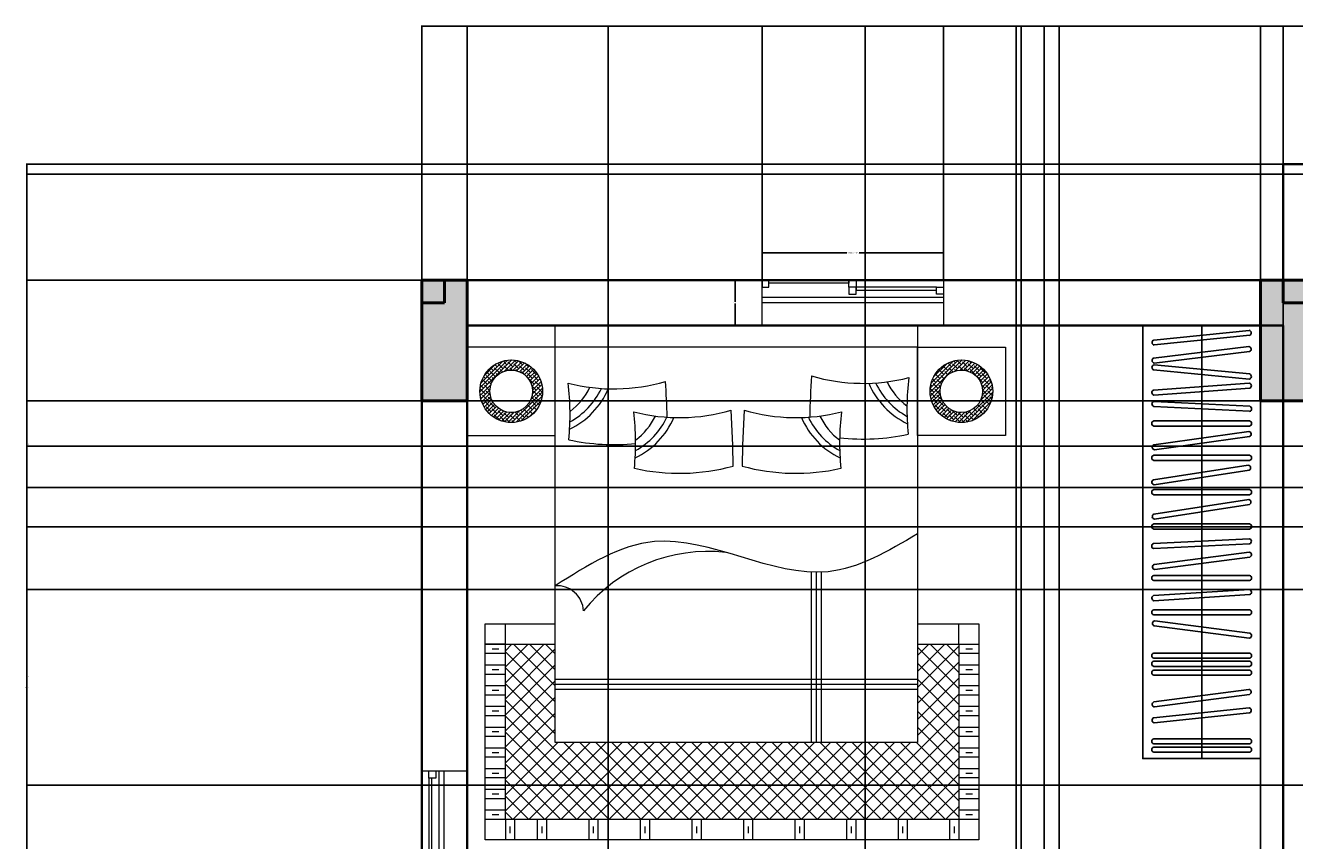
# Model space of a CAD drawing. Units: inches. Extents: x 393 to 993, y 153 to 660.
# Tile 3 of 6: x 393 to 645, y 499 to 660. Entities that reach past the tile are written whole.
import ezdxf

# ---------------------------------------------------------------- set-up
doc = ezdxf.new("R2010")
doc.units = ezdxf.units.IN
doc.header["$MEASUREMENT"] = 0
for name, color, linetype, lineweight in [('A-ANNO-DIMS', 2, 'Continuous', 18), ('A-COLS', 40, 'Continuous', 50), ('A-FLOR-CASE', 72, 'Continuous', 25), ('A-GLAZ', 4, 'Continuous', 20), ('A-WALL', 40, 'Continuous', 35), ('FURNITURE', 72, 'Continuous', 18)]:
    doc.layers.add(name, color=color, linetype=linetype, lineweight=lineweight)
doc.styles.get("Standard").update_dxf_attribs({"font": 'arial.ttf'})
doc.dimstyles.get("Standard").update_dxf_attribs({"dimtxt": 0.18, "dimasz": 0.18, "dimexe": 0.18, "dimexo": 0.0625, "dimgap": 0.09, "dimtad": 0, "dimtih": 1, "dimtoh": 1, "dimdec": 1, "dimzin": 0, "dimdsep": 46, "dimlunit": 3, "dimtxsty": 'Standard', "dimcen": 0.09, "dimadec": 0, "dimazin": 0, "dimtfac": 1, "dimtdec": 1, "dimtofl": 0, "dimtmove": 0, "dimatfit": 3, "dimfxl": 1, "dimtolj": 1, "dimtzin": 0, "dimarcsym": 0})

# ---------------------------------------------------------------- blocks, each defined once
blk = doc.blocks.new('W')
for p, q in [((518.15, 606.48), (554.15, 606.48)), ((518.15, 605.48), (554.15, 605.48))]:
    blk.add_line(p, q)
for points in [[(518.15, 609.91), (554.15, 609.91), (554.15, 600.91), (518.15, 600.91)], [(519.42, 609.91), (518.15, 609.91), (518.15, 608.51), (519.42, 608.51)], [(519.42, 609.91), (535.35, 609.91), (535.35, 609.3), (519.42, 609.3)], [(535.35, 609.91), (536.78, 609.91), (536.78, 608.51), (535.35, 608.51)], [(536.78, 608.51), (535.35, 608.51), (535.35, 607.12), (536.78, 607.12)], [(552.72, 608.51), (536.78, 608.51), (536.78, 607.91), (552.72, 607.91)], [(552.72, 608.51), (554.15, 608.51), (554.15, 607.12), (552.72, 607.12)]]:
    blk.add_lwpolyline(points, close=True)
blk = doc.blocks.new('BED')
h = blk.add_hatch()
h.set_pattern_fill('ANSI38', color=256, scale=4.4)
h.paths.add_polyline_path([(503.33, 587.82, 1), (515.77, 587.82, 1)])
h.paths.add_polyline_path([(513.77, 587.82, -1), (505.33, 587.82, -1)], flags=16)
h = blk.add_hatch()
h.set_pattern_fill('ANSI38', color=256, scale=4.4)
h.paths.add_polyline_path([(592.69, 587.82, 1), (605.13, 587.82, 1)])
h.paths.add_polyline_path([(603.13, 587.82, -1), (594.69, 587.82, -1)], flags=16)
h = blk.add_hatch()
h.set_pattern_fill('ANSI37', color=256, scale=18)
h.paths.add_polyline_path([(518.29, 518.09), (518.29, 537.6), (508.38, 537.6), (508.38, 502.74), (598.4, 502.74), (598.4, 537.6), (590.17, 537.6), (590.17, 518.09)])
for p, q in [((569.1, 551.87), (569.1, 518.09)), ((570.1, 551.87), (570.1, 518.09)), ((571.1, 551.87), (571.1, 518.09)), ((508.38, 537.6), (508.38, 541.6)), ((598.4, 537.6), (598.4, 541.6)), ((508.38, 537.6), (504.38, 537.6)), ((504.38, 537.6), (508.38, 537.6)), ((505.75, 536.69), (507.09, 536.69)), ((598.4, 537.6), (602.4, 537.6)), ((599.77, 536.69), (601.11, 536.69)), ((504.38, 535.78), (508.38, 535.78)), ((598.4, 535.78), (602.4, 535.78)), ((504.38, 533.48), (508.38, 533.48)), ((504.38, 531.66), (508.38, 531.66)), ((505.75, 532.57), (507.09, 532.57)), ((598.4, 533.48), (602.4, 533.48)), ((598.4, 531.66), (602.4, 531.66)), ((599.77, 532.57), (601.11, 532.57)), ((504.38, 529.37), (508.38, 529.37)), ((518.29, 530.67), (590.17, 530.67)), ((518.29, 529.67), (590.17, 529.67)), ((598.4, 529.37), (602.4, 529.37)), ((504.38, 527.54), (508.38, 527.54)), ((505.75, 528.46), (507.09, 528.46)), ((518.29, 528.67), (590.17, 528.67)), ((598.4, 527.54), (602.4, 527.54)), ((599.77, 528.46), (601.11, 528.46)), ((504.38, 525.25), (508.38, 525.25)), ((505.75, 524.34), (507.09, 524.34)), ((598.4, 525.25), (602.4, 525.25)), ((599.77, 524.34), (601.11, 524.34)), ((504.38, 523.43), (508.38, 523.43)), ((598.4, 523.43), (602.4, 523.43)), ((504.38, 521.13), (508.38, 521.13)), ((504.38, 519.31), (508.38, 519.31)), ((505.75, 520.22), (507.09, 520.22)), ((598.4, 521.13), (602.4, 521.13)), ((598.4, 519.31), (602.4, 519.31)), ((599.77, 520.22), (601.11, 520.22)), ((504.38, 517.02), (508.38, 517.02)), ((598.4, 517.02), (602.4, 517.02)), ((504.38, 515.19), (508.38, 515.19)), ((505.75, 516.11), (507.09, 516.11)), ((598.4, 515.19), (602.4, 515.19)), ((599.77, 516.11), (601.11, 516.11)), ((504.38, 512.9), (508.38, 512.9)), ((505.75, 511.99), (507.09, 511.99)), ((598.4, 512.9), (602.4, 512.9)), ((599.77, 511.99), (601.11, 511.99)), ((504.38, 511.08), (508.38, 511.08)), ((598.4, 511.08), (602.4, 511.08)), ((504.38, 508.78), (508.38, 508.78)), ((504.38, 506.96), (508.38, 506.96)), ((505.75, 507.87), (507.09, 507.87)), ((598.4, 508.78), (602.4, 508.78)), ((598.4, 506.96), (602.4, 506.96)), ((599.77, 507.87), (601.11, 507.87)), ((504.38, 504.67), (508.38, 504.67)), ((598.4, 504.67), (602.4, 504.67)), ((504.38, 502.84), (508.38, 502.84)), ((508.38, 502.74), (504.38, 502.74)), ((505.75, 503.76), (507.09, 503.76)), ((508.38, 502.74), (508.38, 498.74)), ((510.2, 502.74), (510.2, 498.74)), ((514.7, 502.74), (514.7, 498.74)), ((516.52, 502.74), (516.52, 498.74)), ((524.93, 502.74), (524.93, 498.74)), ((526.76, 502.74), (526.76, 498.74)), ((535.17, 502.74), (535.17, 498.74)), ((536.99, 502.74), (536.99, 498.74)), ((545.4, 502.74), (545.4, 498.74)), ((547.22, 502.74), (547.22, 498.74)), ((555.64, 502.74), (555.64, 498.74)), ((557.46, 502.74), (557.46, 498.74)), ((565.87, 502.74), (565.87, 498.74)), ((567.69, 502.74), (567.69, 498.74)), ((576.11, 502.74), (576.11, 498.74)), ((577.93, 502.74), (577.93, 498.74)), ((586.34, 502.74), (586.34, 498.74)), ((588.16, 502.74), (588.16, 498.74)), ((596.58, 502.74), (596.58, 498.74)), ((598.4, 502.84), (602.4, 502.84)), ((598.4, 502.74), (598.4, 498.74)), ((599.77, 503.76), (601.11, 503.76)), ((509.29, 501.37), (509.29, 500.03)), ((515.61, 501.37), (515.61, 500.03)), ((525.84, 501.37), (525.84, 500.03)), ((536.08, 501.37), (536.08, 500.03)), ((546.31, 501.37), (546.31, 500.03)), ((556.55, 501.37), (556.55, 500.03)), ((566.78, 501.37), (566.78, 500.03)), ((577.02, 501.37), (577.02, 500.03)), ((587.25, 501.37), (587.25, 500.03)), ((597.49, 501.37), (597.49, 500.03))]:
    blk.add_line(p, q)
for points in [[(518.29, 600.91), (590.17, 600.91), (590.17, 518.09), (518.29, 518.09)], [(518.29, 600.91), (590.17, 600.91), (590.17, 596.58), (518.29, 596.58)], [(518.29, 596.58), (500.81, 596.58), (500.81, 579.05), (518.29, 579.05)], [(590.17, 596.58), (607.65, 596.58), (607.65, 579.05), (590.17, 579.05)]]:
    blk.add_lwpolyline(points, close=True)
for points in [[(590.17, 541.6), (602.4, 541.6), (602.4, 498.74), (504.38, 498.74), (504.38, 541.6), (518.29, 541.6)], [(590.17, 537.6), (598.4, 537.6), (598.4, 502.74), (508.38, 502.74), (508.38, 537.6), (518.29, 537.6)]]:
    blk.add_lwpolyline(points)
for centre, radius in [((509.55, 587.82), 6.22), ((598.91, 587.82), 6.22), ((509.55, 587.82), 4.22), ((598.91, 587.82), 4.22)]:
    blk.add_circle(centre, radius)
for centre, radius, start, end in [((529.91, 624.74), 36.45, 255.5916, 286.3549), ((355.3, 577.59), 185.28, 1.5729, 3.7686), ((754.03, 578.68), 185.28, 176.2314, 178.7587), ((579.42, 625.84), 36.45, 253.6451, 284.4084), ((595.75, 595.21), 12.82, 205.4838, 233.4213), ((639.07, 584.32), 50.97, 172.9945, 185.6503), ((470.26, 583.22), 50.97, 354.3497, 7.0055), ((514.22, 594.55), 15.87, 295.8431, 336.8331), ((514.22, 594.55), 14.59, 298.6055, 334.9463), ((513.58, 594.12), 12.82, 306.5787, 334.5162), ((595.11, 595.65), 15.87, 203.1669, 244.1569), ((595.11, 595.65), 14.59, 205.0537, 241.3945), ((542.93, 619.04), 36.45, 255.5916, 286.3549), ((483.27, 577.52), 50.97, 354.3497, 7.0055), ((527.24, 588.86), 15.87, 295.8431, 336.8331), ((527.24, 588.86), 14.59, 298.6055, 334.9463), ((526.6, 588.42), 12.82, 306.5787, 334.5162), ((368.32, 571.89), 185.28, 0.3263, 3.7686), ((740.67, 571.89), 185.28, 176.2314, 179.6737), ((566.06, 619.04), 36.45, 253.6451, 284.4084), ((581.75, 588.86), 15.87, 203.1669, 244.1569), ((581.75, 588.86), 14.59, 205.0537, 241.3945), ((582.39, 588.42), 12.82, 205.4838, 233.4213), ((625.71, 577.52), 50.97, 172.9945, 185.6503), ((529.89, 618.01), 40.79, 257.3847, 276.1312), ((579.44, 619.11), 40.79, 263.4008, 282.6153), ((542.91, 612.32), 40.79, 257.3847, 285.1893), ((566.08, 612.32), 40.79, 254.8107, 282.6153), ((548.65, 524.17), 31.85, 83.7477, 141.0207), ((518.63, 543.94), 5.27, 2.9325, 93.7021)]:
    blk.add_arc(centre, radius, start, end)
blk.add_open_spline([(590.17, 559.5), (584.37, 556.05), (568.03, 546.36), (541.55, 563.96), (524.71, 553.27), (518.29, 549.19)], degree=3, knots=[0, 0, 0, 0, 19.259502, 54.250447, 75.777559, 75.777559, 75.777559, 75.777559])
blk = doc.blocks.new('COOB')
blk.add_line((626.78, 600.91), (626.78, 514.86))
blk.add_lwpolyline([(638.48, 600.91), (615.08, 600.91), (615.08, 514.86), (638.48, 514.86)], close=True)
for points in [[(636.21, 599.92), (617.25, 598)], [(617.35, 597.01), (636.31, 598.93)], [(636.17, 596.68), (617.24, 594.42)], [(617.36, 593.43), (636.28, 595.69)], [(636.31, 591.25), (617.34, 593.04)], [(617.24, 592.05), (636.21, 590.25)], [(636.24, 589.41), (617.23, 588.06)], [(617.31, 587.07), (636.32, 588.41)], [(617.26, 584.82), (636.29, 583.84)], [(636.35, 584.83), (617.32, 585.82)], [(636.31, 581.92), (617.25, 581.92)], [(617.25, 580.92), (636.31, 580.92)], [(636.15, 579.82), (617.28, 577.19)], [(617.41, 576.2), (636.29, 578.83)], [(636.31, 575.1), (617.25, 575.1)], [(636.04, 573.13), (617.21, 570.23)], [(617.25, 574.1), (636.31, 574.1)], [(617.36, 569.24), (636.2, 572.14)], [(636.31, 568.28), (617.25, 568.28)], [(617.25, 567.28), (636.31, 567.28)], [(636.12, 566.32), (617.28, 563.41)], [(617.44, 562.42), (636.27, 565.34)], [(636.31, 561.46), (617.25, 561.46)], [(617.25, 560.46), (636.31, 560.46)], [(636.25, 558.53), (617.21, 557.57)], [(617.26, 556.57), (636.3, 557.54)], [(636.23, 555.87), (617.33, 553.42)], [(617.46, 552.43), (636.36, 554.88)], [(636.31, 551.24), (617.25, 551.24)], [(617.25, 550.24), (636.31, 550.24)], [(636.26, 548.43), (617.24, 547.23)], [(617.3, 546.23), (636.32, 547.43)], [(636.31, 544.42), (617.25, 544.42)], [(617.25, 543.42), (636.31, 543.42)], [(636.36, 539.77), (617.46, 542.23)], [(617.33, 541.23), (636.23, 538.78)], [(636.31, 535.8), (617.25, 535.8)], [(617.25, 534.8), (636.31, 534.8)], [(636.31, 534.19), (617.25, 534.19)], [(617.25, 533.19), (636.31, 533.19)], [(636.31, 532.44), (617.25, 532.44)], [(617.25, 531.44), (636.31, 531.44)], [(636.16, 528.62), (617.27, 526.12)], [(617.4, 525.13), (636.29, 527.62)], [(636.19, 524.96), (617.24, 522.96)], [(617.35, 521.97), (636.3, 523.96)], [(636.31, 518.8), (617.25, 518.8)], [(617.25, 517.8), (636.31, 517.8)], [(636.31, 517.14), (617.25, 517.14)], [(617.25, 516.14), (636.31, 516.14)]]:
    blk.add_lwpolyline(points)
for centre, start, end in [((636.11, 599.41), 291.987, 79.5876), ((617.44, 597.52), 111.987, 259.5876), ((636.08, 596.17), 293.0233, 80.6239), ((617.43, 592.53), 100.7874, 248.388), ((617.45, 593.94), 113.0233, 260.6239), ((636.12, 590.76), 280.7874, 68.388), ((617.41, 587.58), 110.2473, 257.8479), ((636.13, 588.9), 290.2473, 77.8479), ((617.43, 585.31), 103.2278, 250.8284), ((636.18, 584.34), 283.2278, 70.8284), ((617.4, 581.42), 106.1997, 253.8003), ((636.08, 579.31), 294.1332, 81.7338), ((636.16, 581.42), 286.1997, 73.8003), ((617.49, 576.72), 114.1332, 261.7338), ((617.4, 574.6), 106.1997, 253.8003), ((636.16, 574.6), 286.1997, 73.8003), ((635.98, 572.61), 294.9436, 82.5442), ((617.43, 569.76), 114.9436, 262.5442), ((617.4, 567.78), 106.1997, 253.8003), ((636.16, 567.78), 286.1997, 73.8003), ((636.05, 565.81), 294.9996, 82.6002), ((617.5, 562.94), 114.9996, 262.6002), ((617.4, 560.96), 106.1997, 253.8003), ((636.16, 560.96), 286.1997, 73.8003), ((617.38, 557.08), 109.0898, 256.6904), ((636.13, 558.03), 289.0898, 76.6904), ((636.15, 555.36), 293.5955, 81.1961), ((617.54, 552.94), 113.5955, 261.1961), ((617.4, 550.74), 106.1997, 253.8003), ((636.16, 550.74), 286.1997, 73.8003), ((617.41, 546.74), 109.8088, 257.4094), ((636.14, 547.92), 289.8088, 77.4094), ((617.4, 543.92), 106.1997, 253.8003), ((636.16, 543.92), 286.1997, 73.8003), ((617.54, 541.71), 98.8065, 246.4071), ((636.15, 539.3), 278.8065, 66.4071), ((617.4, 535.3), 106.1997, 253.8003), ((617.4, 533.69), 106.1997, 253.8003), ((636.16, 535.3), 286.1997, 73.8003), ((636.16, 533.69), 286.1997, 73.8003), ((617.4, 531.94), 106.1997, 253.8003), ((636.16, 531.94), 286.1997, 73.8003), ((636.08, 528.1), 293.7284, 81.329), ((617.48, 525.64), 113.7284, 261.329), ((636.1, 524.44), 292.2058, 79.8064), ((617.44, 522.48), 112.2058, 259.8064), ((617.4, 518.3), 106.1997, 253.8003), ((617.4, 516.64), 106.1997, 253.8003), ((636.16, 518.3), 286.1997, 73.8003), ((636.16, 516.64), 286.1997, 73.8003)]:
    blk.add_arc(centre, 0.521, start, end)
blk = doc.blocks.new('COL-9X24-RH')
h = blk.add_hatch(color=256)
h.dxf.hatch_style = 1
h.paths.add_polyline_path([(4.5, 19.5), (4.5, 24), (0, 24), (0, 0), (9, 0), (9, 19.5)])
h = blk.add_hatch(color=256)
h.dxf.hatch_style = 1
h.paths.add_polyline_path([(4.5, 19.5), (9, 19.5), (9, 24), (4.5, 24)])
for p, q in [((4.5, 24), (4.5, 19.5)), ((4.5, 24), (9, 24)), ((9, 24), (9, 19.5)), ((4.5, 19.5), (9, 19.5))]:
    blk.add_line(p, q)
blk.add_lwpolyline([(0, 24), (9, 24), (9, 0), (0, 0), (0, 24)])
blk = doc.blocks.new('COL-9X24-LH')
h = blk.add_hatch(color=256)
h.dxf.hatch_style = 1
h.paths.add_polyline_path([(4.5, 24), (0, 24), (0, 19.5), (4.5, 19.5)])
h = blk.add_hatch(color=256)
h.dxf.hatch_style = 1
h.paths.add_polyline_path([(4.5, 19.5), (0, 19.5), (0, 0), (9, 0), (9, 24), (4.5, 24)])
for p, q in [((4.5, 24), (0, 24)), ((0, 24), (0, 19.5)), ((4.5, 24), (4.5, 19.5)), ((4.5, 19.5), (0, 19.5))]:
    blk.add_line(p, q)
blk.add_lwpolyline([(9, 24), (0, 24), (0, 0), (9, 0), (9, 24)])
blk = doc.blocks.new('*D24')
at = {"layer": 'A-ANNO-DIMS', "color": 0, "lineweight": -2, "transparency": 16777216}
for p, q in [((539.56, 609.97), (539.56, 615.49)), ((539.74, 615.31), (556.32, 615.31)), ((575.38, 615.31), (558.8, 615.31)), ((575.56, 609.97), (575.56, 615.49))]:
    blk.add_line(p, q, dxfattribs=at)
at = {"layer": 'A-ANNO-DIMS', "color": 0, "transparency": 16777216}
for points in [[(539.74, 615.34), (539.74, 615.28), (539.56, 615.31)], [(575.38, 615.34), (575.38, 615.28), (575.56, 615.31)]]:
    blk.add_solid(points, dxfattribs=at)
at = {"layer": 'Defpoints', "color": 0, "transparency": 16777216}
for p in [(575.56, 615.31), (539.56, 609.91), (575.56, 609.91)]:
    blk.add_point(p, dxfattribs=at)
at = {"layer": 'A-ANNO-DIMS', "color": 0, "transparency": 16777216, "insert": (557.56, 615.31), "char_height": 0.18, "attachment_point": 5}
blk.add_mtext('\\A1;WINDOW A 36 TYP.', dxfattribs=at)
blk = doc.blocks.new('*D25')
at = {"layer": 'A-ANNO-DIMS', "color": 0, "lineweight": -2, "transparency": 16777216}
for p, q in [((539.5, 609.91), (533.98, 609.91)), ((534.16, 609.73), (534.16, 605.59)), ((534.16, 601.09), (534.16, 605.22)), ((539.5, 600.91), (533.98, 600.91))]:
    blk.add_line(p, q, dxfattribs=at)
at = {"layer": 'A-ANNO-DIMS', "color": 0, "transparency": 16777216}
for points in [[(534.13, 609.73), (534.19, 609.73), (534.16, 609.91)], [(534.13, 601.09), (534.19, 601.09), (534.16, 600.91)]]:
    blk.add_solid(points, dxfattribs=at)
at = {"layer": 'Defpoints', "color": 0, "transparency": 16777216}
for p in [(534.16, 609.91), (539.56, 609.91), (539.56, 600.91)]:
    blk.add_point(p, dxfattribs=at)
at = {"layer": 'A-ANNO-DIMS', "color": 0, "transparency": 16777216, "insert": (534.16, 605.41), "char_height": 0.18, "attachment_point": 5}
blk.add_mtext('\\A1;9 TYP.', dxfattribs=at)
blk = doc.blocks.new('*D46')
at = {"layer": 'A-ANNO-DIMS', "color": 0, "lineweight": -2, "transparency": 16777216}
for p, q in [((471.98, 609.97), (471.98, 660.49)), ((472.16, 660.31), (505.38, 660.31)), ((539.38, 660.31), (506.16, 660.31)), ((539.56, 609.97), (539.56, 660.49))]:
    blk.add_line(p, q, dxfattribs=at)
at = {"layer": 'A-ANNO-DIMS', "color": 0, "transparency": 16777216}
for points in [[(472.16, 660.34), (472.16, 660.28), (471.98, 660.31)], [(539.38, 660.34), (539.38, 660.28), (539.56, 660.31)]]:
    blk.add_solid(points, dxfattribs=at)
at = {"layer": 'Defpoints', "color": 0, "transparency": 16777216}
for p in [(539.56, 660.31), (471.98, 609.91), (539.56, 609.91)]:
    blk.add_point(p, dxfattribs=at)
at = {"layer": 'A-ANNO-DIMS', "color": 0, "transparency": 16777216, "insert": (505.77, 660.31), "char_height": 0.18, "attachment_point": 5}
blk.add_mtext('\\A1;67.58', dxfattribs=at)
blk = doc.blocks.new('*D47')
at = {"layer": 'A-ANNO-DIMS', "color": 0, "lineweight": -2, "transparency": 16777216}
for p, q in [((575.56, 609.97), (575.56, 660.49)), ((575.74, 660.31), (608.88, 660.31)), ((642.8, 660.31), (609.66, 660.31)), ((642.98, 609.97), (642.98, 660.49))]:
    blk.add_line(p, q, dxfattribs=at)
at = {"layer": 'A-ANNO-DIMS', "color": 0, "transparency": 16777216}
for points in [[(575.74, 660.34), (575.74, 660.28), (575.56, 660.31)], [(642.8, 660.34), (642.8, 660.28), (642.98, 660.31)]]:
    blk.add_solid(points, dxfattribs=at)
at = {"layer": 'Defpoints', "color": 0, "transparency": 16777216}
for p in [(642.98, 660.31), (575.56, 609.91), (642.98, 609.91)]:
    blk.add_point(p, dxfattribs=at)
at = {"layer": 'A-ANNO-DIMS', "color": 0, "transparency": 16777216, "insert": (609.27, 660.31), "char_height": 0.18, "attachment_point": 5}
blk.add_mtext('\\A1;67.42', dxfattribs=at)
blk = doc.blocks.new('*D48')
at = {"layer": 'A-ANNO-DIMS', "color": 0, "lineweight": -2, "transparency": 16777216}
for p, q in [((642.98, 632.97), (642.98, 660.49)), ((643.16, 660.31), (719.2, 660.31)), ((795.8, 660.31), (719.76, 660.31)), ((795.98, 632.97), (795.98, 660.49))]:
    blk.add_line(p, q, dxfattribs=at)
at = {"layer": 'A-ANNO-DIMS', "color": 0, "transparency": 16777216}
for points in [[(643.16, 660.34), (643.16, 660.28), (642.98, 660.31)], [(795.8, 660.34), (795.8, 660.28), (795.98, 660.31)]]:
    blk.add_solid(points, dxfattribs=at)
at = {"layer": 'Defpoints', "color": 0, "transparency": 16777216}
for p in [(795.98, 660.31), (642.98, 632.91), (795.98, 632.91)]:
    blk.add_point(p, dxfattribs=at)
at = {"layer": 'A-ANNO-DIMS', "color": 0, "transparency": 16777216, "insert": (719.48, 660.31), "char_height": 0.18, "attachment_point": 5}
blk.add_mtext('\\A1;153', dxfattribs=at)
blk = doc.blocks.new('*D54')
at = {"layer": 'A-ANNO-DIMS', "color": 0, "lineweight": -2, "transparency": 16777216}
for p, q in [((471.92, 609.91), (393.4, 609.91)), ((393.58, 609.73), (393.58, 531.34)), ((393.58, 452.59), (393.58, 530.97)), ((471.92, 452.41), (393.4, 452.41))]:
    blk.add_line(p, q, dxfattribs=at)
at = {"layer": 'A-ANNO-DIMS', "color": 0, "transparency": 16777216}
for points in [[(393.55, 609.73), (393.61, 609.73), (393.58, 609.91)], [(393.55, 452.59), (393.61, 452.59), (393.58, 452.41)]]:
    blk.add_solid(points, dxfattribs=at)
at = {"layer": 'Defpoints', "color": 0, "transparency": 16777216}
for p in [(393.58, 609.91), (471.98, 609.91), (471.98, 452.41)]:
    blk.add_point(p, dxfattribs=at)
at = {"layer": 'A-ANNO-DIMS', "color": 0, "transparency": 16777216, "insert": (393.58, 531.16), "char_height": 0.18, "attachment_point": 5}
blk.add_mtext('\\A1;157.5', dxfattribs=at)
blk = doc.blocks.new('*D55')
at = {"layer": 'A-ANNO-DIMS', "color": 0, "lineweight": -2, "transparency": 16777216}
for p, q in [((791.42, 630.91), (393.4, 630.91)), ((393.58, 630.73), (393.58, 596.09)), ((393.58, 561.09), (393.58, 595.72)), ((791.42, 560.91), (393.4, 560.91))]:
    blk.add_line(p, q, dxfattribs=at)
at = {"layer": 'A-ANNO-DIMS', "color": 0, "transparency": 16777216}
for points in [[(393.55, 630.73), (393.61, 630.73), (393.58, 630.91)], [(393.55, 561.09), (393.61, 561.09), (393.58, 560.91)]]:
    blk.add_solid(points, dxfattribs=at)
at = {"layer": 'Defpoints', "color": 0, "transparency": 16777216}
for p in [(791.48, 630.91), (393.58, 560.91), (791.48, 560.91)]:
    blk.add_point(p, dxfattribs=at)
at = {"layer": 'A-ANNO-DIMS', "color": 0, "transparency": 16777216, "insert": (393.58, 595.91), "char_height": 0.18, "attachment_point": 5}
blk.add_mtext('\\A1;70', dxfattribs=at)
blk = doc.blocks.new('*D56')
at = {"layer": 'A-ANNO-DIMS', "color": 0, "lineweight": -2, "transparency": 16777216}
for p, q in [((480.98, 397.47), (480.98, 660.49)), ((481.16, 660.31), (535.7, 660.31)), ((590.8, 660.31), (536.26, 660.31)), ((590.98, 397.47), (590.98, 660.49))]:
    blk.add_line(p, q, dxfattribs=at)
at = {"layer": 'A-ANNO-DIMS', "color": 0, "transparency": 16777216}
for points in [[(481.16, 660.34), (481.16, 660.28), (480.98, 660.31)], [(590.8, 660.34), (590.8, 660.28), (590.98, 660.31)]]:
    blk.add_solid(points, dxfattribs=at)
at = {"layer": 'Defpoints', "color": 0, "transparency": 16777216}
for p in [(590.98, 660.31), (480.98, 397.41), (590.98, 397.41)]:
    blk.add_point(p, dxfattribs=at)
at = {"layer": 'A-ANNO-DIMS', "color": 0, "transparency": 16777216, "insert": (535.98, 660.31), "char_height": 0.18, "attachment_point": 5}
blk.add_mtext('\\A1;110', dxfattribs=at)
blk = doc.blocks.new('*D61')
at = {"layer": 'A-ANNO-DIMS', "color": 0, "lineweight": -2, "transparency": 16777216}
for p, q in [((559.98, 452.47), (559.98, 660.49)), ((560.16, 660.31), (574.76, 660.31)), ((589.8, 660.31), (575.2, 660.31)), ((589.98, 452.47), (589.98, 660.49))]:
    blk.add_line(p, q, dxfattribs=at)
at = {"layer": 'A-ANNO-DIMS', "color": 0, "transparency": 16777216}
for points in [[(560.16, 660.34), (560.16, 660.28), (559.98, 660.31)], [(589.8, 660.34), (589.8, 660.28), (589.98, 660.31)]]:
    blk.add_solid(points, dxfattribs=at)
at = {"layer": 'Defpoints', "color": 0, "transparency": 16777216}
for p in [(589.98, 660.31), (559.98, 452.41), (589.98, 452.41)]:
    blk.add_point(p, dxfattribs=at)
at = {"layer": 'A-ANNO-DIMS', "color": 0, "transparency": 16777216, "insert": (574.98, 660.31), "char_height": 0.18, "attachment_point": 5}
blk.add_mtext('\\A1;30', dxfattribs=at)
blk = doc.blocks.new('*D64')
at = {"layer": 'A-ANNO-DIMS', "color": 0, "lineweight": -2, "transparency": 16777216}
for p, q in [((932.42, 576.91), (393.4, 576.91)), ((393.58, 576.73), (393.58, 529.09)), ((393.58, 481.09), (393.58, 528.72)), ((932.42, 480.91), (393.4, 480.91))]:
    blk.add_line(p, q, dxfattribs=at)
at = {"layer": 'A-ANNO-DIMS', "color": 0, "transparency": 16777216}
for points in [[(393.55, 576.73), (393.61, 576.73), (393.58, 576.91)], [(393.55, 481.09), (393.61, 481.09), (393.58, 480.91)]]:
    blk.add_solid(points, dxfattribs=at)
at = {"layer": 'Defpoints', "color": 0, "transparency": 16777216}
for p in [(393.58, 576.91), (932.48, 576.91), (932.48, 480.91)]:
    blk.add_point(p, dxfattribs=at)
at = {"layer": 'A-ANNO-DIMS', "color": 0, "transparency": 16777216, "insert": (393.58, 528.91), "char_height": 0.18, "attachment_point": 5}
blk.add_mtext('\\A1;96', dxfattribs=at)
blk = doc.blocks.new('*D65')
at = {"layer": 'A-ANNO-DIMS', "color": 0, "lineweight": -2, "transparency": 16777216}
for p, q in [((598.48, 456.97), (598.48, 660.49)), ((598.66, 660.31), (618.26, 660.31)), ((638.3, 660.31), (618.7, 660.31)), ((638.48, 458.47), (638.48, 660.49))]:
    blk.add_line(p, q, dxfattribs=at)
at = {"layer": 'A-ANNO-DIMS', "color": 0, "transparency": 16777216}
for points in [[(598.66, 660.34), (598.66, 660.28), (598.48, 660.31)], [(638.3, 660.34), (638.3, 660.28), (638.48, 660.31)]]:
    blk.add_solid(points, dxfattribs=at)
at = {"layer": 'Defpoints', "color": 0, "transparency": 16777216}
for p in [(638.48, 660.31), (598.48, 456.91), (638.48, 458.41)]:
    blk.add_point(p, dxfattribs=at)
at = {"layer": 'A-ANNO-DIMS', "color": 0, "transparency": 16777216, "insert": (618.48, 660.31), "char_height": 0.18, "attachment_point": 5}
blk.add_mtext('\\A1;40', dxfattribs=at)
blk = doc.blocks.new('*D66')
at = {"layer": 'A-ANNO-DIMS', "color": 0, "lineweight": -2, "transparency": 16777216}
for p, q in [((642.92, 632.91), (393.4, 632.91)), ((393.58, 632.73), (393.58, 621.59)), ((393.58, 610.09), (393.58, 621.22)), ((642.92, 609.91), (393.4, 609.91))]:
    blk.add_line(p, q, dxfattribs=at)
at = {"layer": 'A-ANNO-DIMS', "color": 0, "transparency": 16777216}
for points in [[(393.55, 632.73), (393.61, 632.73), (393.58, 632.91)], [(393.55, 610.09), (393.61, 610.09), (393.58, 609.91)]]:
    blk.add_solid(points, dxfattribs=at)
at = {"layer": 'Defpoints', "color": 0, "transparency": 16777216}
for p in [(393.58, 632.91), (642.98, 632.91), (642.98, 609.91)]:
    blk.add_point(p, dxfattribs=at)
at = {"layer": 'A-ANNO-DIMS', "color": 0, "transparency": 16777216, "insert": (393.58, 621.41), "char_height": 0.18, "attachment_point": 5}
blk.add_mtext('\\A1;23', dxfattribs=at)
blk = doc.blocks.new('*D74')
at = {"layer": 'A-ANNO-DIMS', "color": 0, "lineweight": -2, "transparency": 16777216}
for p, q in [((956.42, 585.91), (393.4, 585.91)), ((393.58, 585.73), (393.58, 577.48)), ((393.58, 568.88), (393.58, 577.12)), ((956.42, 568.7), (393.4, 568.7))]:
    blk.add_line(p, q, dxfattribs=at)
at = {"layer": 'A-ANNO-DIMS', "color": 0, "transparency": 16777216}
for points in [[(393.55, 585.73), (393.61, 585.73), (393.58, 585.91)], [(393.55, 568.88), (393.61, 568.88), (393.58, 568.7)]]:
    blk.add_solid(points, dxfattribs=at)
at = {"layer": 'Defpoints', "color": 0, "transparency": 16777216}
for p in [(393.58, 585.91), (956.48, 585.91), (956.48, 568.7)]:
    blk.add_point(p, dxfattribs=at)
at = {"layer": 'A-ANNO-DIMS', "color": 0, "transparency": 16777216, "insert": (393.58, 577.3), "char_height": 0.18, "attachment_point": 5}
blk.add_mtext('\\A1;17.21', dxfattribs=at)
blk = doc.blocks.new('*D77')
at = {"layer": 'A-ANNO-DIMS', "color": 0, "lineweight": -2, "transparency": 16777216}
for p, q in [((595.48, 397.47), (595.48, 660.49)), ((595.66, 660.31), (618.9, 660.31)), ((642.8, 660.31), (619.56, 660.31)), ((642.98, 392.97), (642.98, 660.49))]:
    blk.add_line(p, q, dxfattribs=at)
at = {"layer": 'A-ANNO-DIMS', "color": 0, "transparency": 16777216}
for points in [[(595.66, 660.34), (595.66, 660.28), (595.48, 660.31)], [(642.8, 660.34), (642.8, 660.28), (642.98, 660.31)]]:
    blk.add_solid(points, dxfattribs=at)
at = {"layer": 'Defpoints', "color": 0, "transparency": 16777216}
for p in [(642.98, 660.31), (595.48, 397.41), (642.98, 392.91)]:
    blk.add_point(p, dxfattribs=at)
at = {"layer": 'A-ANNO-DIMS', "color": 0, "transparency": 16777216, "insert": (619.23, 660.31), "char_height": 0.18, "attachment_point": 5}
blk.add_mtext('\\A1;47.5', dxfattribs=at)
blk = doc.blocks.new('*D79')
at = {"layer": 'A-ANNO-DIMS', "color": 0, "lineweight": -2, "transparency": 16777216}
for p, q in [((480.98, 378.39), (480.98, 660.49)), ((481.16, 660.31), (494.76, 660.31)), ((508.8, 660.31), (495.2, 660.31)), ((508.98, 367.89), (508.98, 660.49))]:
    blk.add_line(p, q, dxfattribs=at)
at = {"layer": 'A-ANNO-DIMS', "color": 0, "transparency": 16777216}
for points in [[(481.16, 660.34), (481.16, 660.28), (480.98, 660.31)], [(508.8, 660.34), (508.8, 660.28), (508.98, 660.31)]]:
    blk.add_solid(points, dxfattribs=at)
at = {"layer": 'Defpoints', "color": 0, "transparency": 16777216}
for p in [(508.98, 660.31), (480.98, 378.32), (508.98, 367.82)]:
    blk.add_point(p, dxfattribs=at)
at = {"layer": 'A-ANNO-DIMS', "color": 0, "transparency": 16777216, "insert": (494.98, 660.31), "char_height": 0.18, "attachment_point": 5}
blk.add_mtext('\\A1;28', dxfattribs=at)
blk = doc.blocks.new('*D84')
at = {"layer": 'A-ANNO-DIMS', "color": 0, "lineweight": -2, "transparency": 16777216}
for p, q in [((956.42, 548.43), (393.4, 548.43)), ((393.58, 548.25), (393.58, 529.18)), ((393.58, 509.74), (393.58, 528.81)), ((956.42, 509.56), (393.4, 509.56))]:
    blk.add_line(p, q, dxfattribs=at)
at = {"layer": 'A-ANNO-DIMS', "color": 0, "transparency": 16777216}
for points in [[(393.55, 548.25), (393.61, 548.25), (393.58, 548.43)], [(393.55, 509.74), (393.61, 509.74), (393.58, 509.56)]]:
    blk.add_solid(points, dxfattribs=at)
at = {"layer": 'Defpoints', "color": 0, "transparency": 16777216}
for p in [(393.58, 548.43), (956.48, 548.43), (956.48, 509.56)]:
    blk.add_point(p, dxfattribs=at)
at = {"layer": 'A-ANNO-DIMS', "color": 0, "transparency": 16777216, "insert": (393.58, 529), "char_height": 0.18, "attachment_point": 5}
blk.add_mtext('\\A1;38.87', dxfattribs=at)

msp = doc.modelspace()

# ---------------------------------------------------------------- linework, layer by layer
at = {"layer": 'A-WALL'}
for p, q in [((642.9798, 632.9066), (642.9798, 609.9066)), ((642.9798, 632.9066), (795.9798, 632.9066)), ((471.9798, 609.9066), (471.9798, 180.9066)), ((471.9798, 609.9066), (642.9798, 609.9066)), ((480.9798, 600.9066), (480.9798, 456.9066)), ((480.9798, 600.9066), (642.9798, 600.9066)), ((642.9798, 600.9066), (642.9798, 476.4066))]:
    msp.add_line(p, q, dxfattribs=at)

# ---------------------------------------------------------------- block references
at = {"layer": 'A-COLS'}
for name, p in [('COL-9X24-LH', (471.98, 585.907)), ('COL-9X24-RH', (638.48, 585.907))]:
    msp.add_blockref(name, p, dxfattribs=at)
at = {"layer": 'A-FLOR-CASE'}
msp.add_blockref('COOB', (0, 0), dxfattribs=at)
at = {"layer": 'A-GLAZ'}
msp.add_blockref('W', (21.4113, 0), dxfattribs=at)
at = {"layer": 'A-GLAZ', "rotation": 90}
msp.add_blockref('W', (1081.8865, -41.7421), dxfattribs=at)
at = {"layer": 'FURNITURE'}
msp.add_blockref('BED', (-19.8291, 0), dxfattribs=at)

# ---------------------------------------------------------------- dimensions: what is measured, and where the dimension line sits
at = {"layer": 'A-ANNO-DIMS'}
for base, p1, p2, override, picture, middle in [((539.56, 660.3066), (471.9798, 609.9066), (539.56, 609.9066), {"dimdec": 2, "dimlfac": 1, "dimrnd": 0, "dimzin": 0, "dimdsep": 46, "dimlunit": 2}, '*D46', (505.7699, 660.3066)), ((590.9798, 660.3066), (480.9798, 397.4066), (590.9798, 397.4066), {"dimdec": 0, "dimlfac": 1, "dimrnd": 0, "dimzin": 0, "dimdsep": 46, "dimlunit": 2}, '*D56', (535.9798, 660.3066)), ((508.9798, 660.3066), (480.9798, 378.3225), (508.9798, 367.8226), {"dimdec": 0, "dimlfac": 1, "dimrnd": 0, "dimzin": 0, "dimdsep": 46, "dimlunit": 2}, '*D79', (494.9798, 660.3066)), ((589.9798, 660.3066), (559.9798, 452.4066), (589.9798, 452.4066), {"dimdec": 0, "dimlfac": 1, "dimrnd": 0, "dimzin": 0, "dimdsep": 46, "dimlunit": 2}, '*D61', (574.9798, 660.3066)), ((642.9798, 660.3066), (575.56, 609.9066), (642.9798, 609.9066), {"dimdec": 2, "dimlfac": 1, "dimrnd": 0, "dimzin": 0, "dimdsep": 46, "dimlunit": 2}, '*D47', (609.2699, 660.3066)), ((642.9798, 660.3066), (595.4798, 397.4066), (642.9798, 392.9066), {"dimdec": 1, "dimlfac": 1, "dimrnd": 0, "dimzin": 0, "dimdsep": 46, "dimlunit": 2}, '*D77', (619.2298, 660.3066)), ((638.4798, 660.3066), (598.4798, 456.9066), (638.4798, 458.4066), {"dimdec": 0, "dimlfac": 1, "dimrnd": 0, "dimzin": 0, "dimdsep": 46, "dimlunit": 2}, '*D65', (618.4798, 660.3066)), ((795.9798, 660.3066), (642.9798, 632.9066), (795.9798, 632.9066), {"dimdec": 0, "dimlfac": 1, "dimrnd": 0, "dimzin": 0, "dimdsep": 46, "dimlunit": 2}, '*D48', (719.4798, 660.3066))]:
    dim = msp.add_linear_dim(base=base, p1=p1, p2=p2, dimstyle='Standard', override=override, dxfattribs=at)
    dim.commit()
    dim.dimension.update_dxf_attribs({"geometry": picture, "text_midpoint": middle})
for base, p1, p2, override, picture, middle in [((393.5798, 632.9066), (642.9798, 609.9066), (642.9798, 632.9066), {"dimdec": 0, "dimlfac": 1, "dimrnd": 0, "dimzin": 0, "dimdsep": 46, "dimlunit": 2}, '*D66', (393.5798, 621.4066)), ((393.5798, 560.9066), (791.4798, 630.9066), (791.4798, 560.9066), {"dimdec": 0, "dimlfac": 1, "dimrnd": 0, "dimzin": 0, "dimdsep": 46, "dimlunit": 2}, '*D55', (393.5798, 595.9066)), ((393.5798, 609.9066), (471.9798, 452.4066), (471.9798, 609.9066), {"dimdec": 1, "dimlfac": 1, "dimrnd": 0, "dimzin": 0, "dimdsep": 46, "dimlunit": 2}, '*D54', (393.5798, 531.1566)), ((393.5798, 585.9066), (956.4798, 568.6983), (956.4798, 585.9066), {"dimdec": 2, "dimlfac": 1, "dimrnd": 0, "dimzin": 0, "dimdsep": 46, "dimlunit": 2}, '*D74', (393.5798, 577.3025)), ((393.5798, 576.9066), (932.4798, 480.9066), (932.4798, 576.9066), {"dimdec": 0, "dimlfac": 1, "dimrnd": 0, "dimzin": 0, "dimdsep": 46, "dimlunit": 2}, '*D64', (393.5798, 528.9066)), ((393.5798, 548.43), (956.4798, 509.5613), (956.4798, 548.43), {"dimdec": 2, "dimlfac": 1, "dimrnd": 0, "dimzin": 0, "dimdsep": 46, "dimlunit": 2}, '*D84', (393.5798, 528.9957))]:
    dim = msp.add_linear_dim(base=base, p1=p1, p2=p2, angle=90, dimstyle='Standard', override=override, dxfattribs=at)
    dim.commit()
    dim.dimension.update_dxf_attribs({"geometry": picture, "text_midpoint": middle})
dim = msp.add_linear_dim(base=(575.56, 615.3066), p1=(539.56, 609.9066), p2=(575.56, 609.9066), text='WINDOW A <> TYP.', dimstyle='Standard', override={"dimdec": 0, "dimlfac": 1, "dimrnd": 0, "dimzin": 0, "dimdsep": 46, "dimlunit": 2}, dxfattribs=at)
dim.commit()
dim.dimension.update_dxf_attribs({"geometry": '*D24', "text_midpoint": (557.56, 615.3066)})
dim = msp.add_linear_dim(base=(534.16, 609.9066), p1=(539.56, 600.9066), p2=(539.56, 609.9066), angle=90, text='<> TYP.', dimstyle='Standard', override={"dimdec": 0, "dimlfac": 1, "dimrnd": 0, "dimzin": 0, "dimdsep": 46, "dimlunit": 2}, dxfattribs=at)
dim.commit()
dim.dimension.update_dxf_attribs({"geometry": '*D25', "text_midpoint": (534.16, 605.4066)})

doc.saveas('drawing.dxf')
